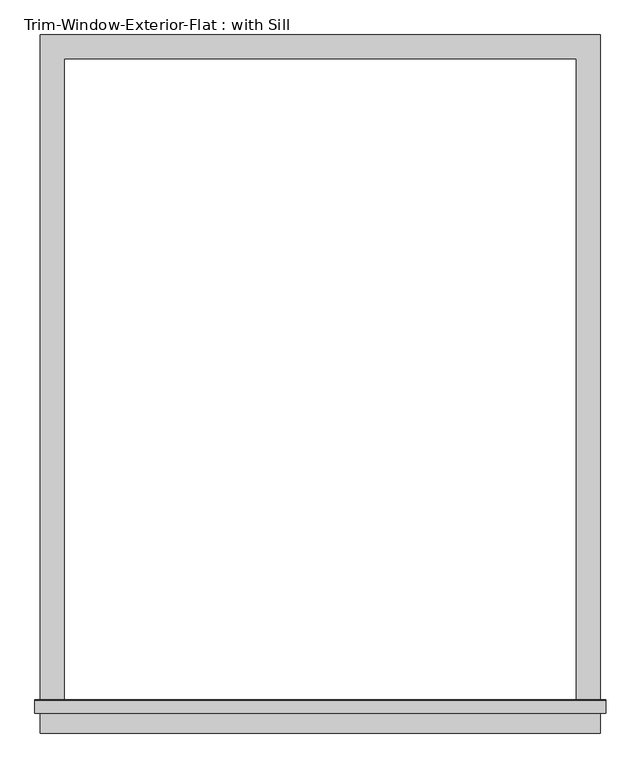
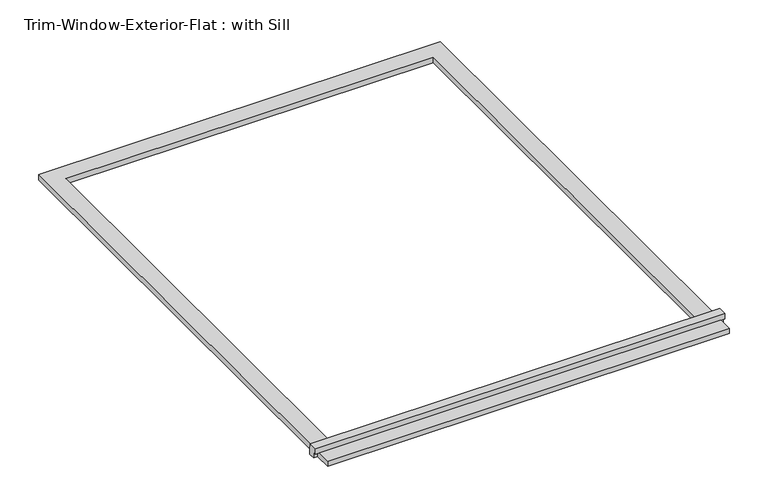
"""IFC4 building model written with IfcOpenShell, lengths in millimetres: proxy geometry, Trim-Window-Exterior-Flat : with Sill."""

from ifc_helpers import new_model, si_unit, frame, origin, origin_with_axes, place, context, project, spatial, polyline, outline, extrude, source, transform, mapped, element, save


def trim_window_exterior_flat_with_sill_92b9b949(model_context):
    return source(origin(), model_context, "Body", "SweptSolid", [
        extrude(outline(polyline([(666.75, -1546.1823709), (666.75, -1603.3323709), (-666.75, -1603.3323709), (-666.75, -1546.1823709), (666.75, -1546.1823709)])), origin_with_axes(), (0.0, 0.0, 1.0), 19.05),
        extrude(outline(polyline([(-1555.75, 38.1), (-1526.4580645, 38.1), (-1524.0, 19.05), (-1524.0, 0.0), (-1546.1823709, 0.0), (-1546.1823709, 19.05), (-1555.75, 19.05), (-1555.75, 38.1)])), frame((-679.45, 0.0, 0.0), z_axis=(1.0, 0.0, 0.0), x_axis=(0.0, 1.0, 0.0)), (0.0, 0.0, 1.0), 1358.9),
        extrude(outline(polyline([(-666.75, 57.15), (666.75, 57.15), (666.75, -1524.0), (609.6, -1524.0), (609.6, 0.0), (-609.6, 0.0), (-609.6, -1524.0), (-666.75, -1524.0), (-666.75, 57.15)])), origin_with_axes(), (0.0, 0.0, 1.0), 19.05),
    ])


if __name__ == "__main__":
    model = new_model("IFC4")
    model_context = context("Model", 3, world=origin())
    ifc_project = project(units=[si_unit("LENGTHUNIT", "METRE", prefix="MILLI")], contexts=[model_context])
    site = spatial("IfcSite", under=ifc_project)
    building = spatial("IfcBuilding", under=site)
    placement = place(None, origin())
    trim_window_exterior_flat_with_sill_shape = trim_window_exterior_flat_with_sill_92b9b949(model_context)
    element("IfcBuildingElementProxy", 1, Name="Trim-Window-Exterior-Flat : with Sill", ObjectType="Trim-Window-Exterior-Flat : with Sill", at=placement, inside=building, context=model_context, shape_type="MappedRepresentation", body=[
        mapped(trim_window_exterior_flat_with_sill_shape, transform((0.0, 0.0, 0.0), x_axis=(1.0, 0.0, 0.0), y_axis=(0.0, 1.0, 0.0), z_axis=(0.0, 0.0, 1.0))),
    ])
    save(model, "model.ifc")

# Revit data of these elements
# Type "Trim-Window-Exterior-Flat : with Sill"
#   Trim Width = 0' - 2 1/4"
#   Trim Thickness_Picture Frame = 0' - 1 1/4"
#   Trim Thickness_with Sill = 0' - 0 3/4"
#   Sill Thickness = 0' - 1 1/4"
#   Opening Width [instance default] = 2' - 0"
#   Opening Height [instance default] = 3' - 0"
#   Default Elevation = 4' - 0"
#   Sill = yes
#   Picture Frame = no
#   Trim Material [instance default] = none
# Element 1 (IfcBuildingElementProxy, "Trim-Window-Exterior-Flat : with Sill")
#   Opening Width = 4' - 0"
#   Opening Height = 5' - 0"
#   Trim Material = Clad - White
#   Materials on its faces: "Clad - White"
# Materials
#   "Clad - White": class "Wood", colour RGB 245 245 243, transparency 0, Cost = 0
